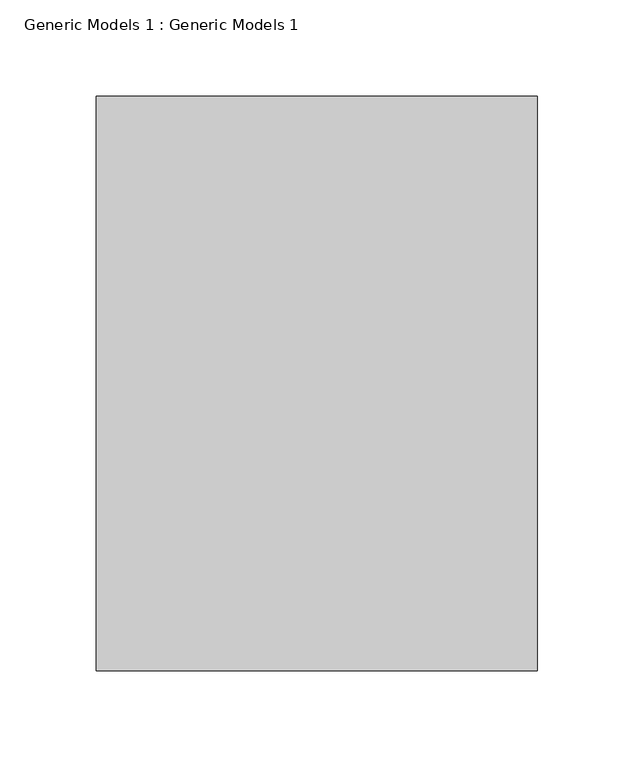
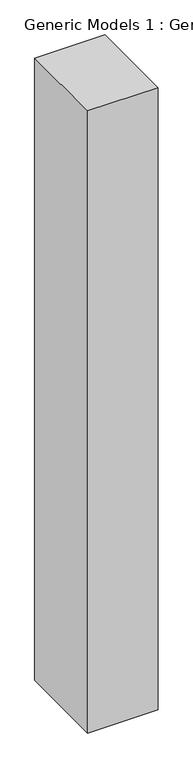
"""IFC4 building model written with IfcOpenShell, lengths in millimetres: proxy geometry, Generic Models 1 : Generic Models 1."""

from ifc_helpers import new_model, si_unit, frame, origin, place, context, project, spatial, polyline, outline, extrude, source, transform, mapped, element, save


def generic_models_1_generic_models_1_9fbe4478(model_context):
    return source(origin(), model_context, "Body", "SweptSolid", [
        extrude(outline(polyline([(375.7271331, -11975.7643494), (147.1271331, -11975.7643494), (147.1271331, -11677.9324242), (375.7271331, -11677.9324242), (375.7271331, -11975.7643494)])), frame((0.0, 0.0, 457.2), z_axis=(0.0, 0.0, 1.0), x_axis=(1.0, 0.0, 0.0)), (0.0, 0.0, 1.0), 2133.6),
    ])


if __name__ == "__main__":
    model = new_model("IFC4")
    model_context = context("Model", 3, world=origin())
    ifc_project = project(units=[si_unit("LENGTHUNIT", "METRE", prefix="MILLI")], contexts=[model_context])
    site = spatial("IfcSite", under=ifc_project)
    building = spatial("IfcBuilding", under=site)
    placement = place(None, origin())
    generic_models_1_generic_models_1_shape = generic_models_1_generic_models_1_9fbe4478(model_context)
    element("IfcBuildingElementProxy", 1, Name="Generic Models 1 : Generic Models 1", ObjectType="Generic Models 1 : Generic Models 1", at=placement, inside=building, context=model_context, shape_type="MappedRepresentation", body=[
        mapped(generic_models_1_generic_models_1_shape, transform((0.0, 0.0, 0.0), x_axis=(1.0, 0.0, 0.0), y_axis=(0.0, 1.0, 0.0), z_axis=(0.0, 0.0, 1.0))),
    ])
    save(model, "model.ifc")
